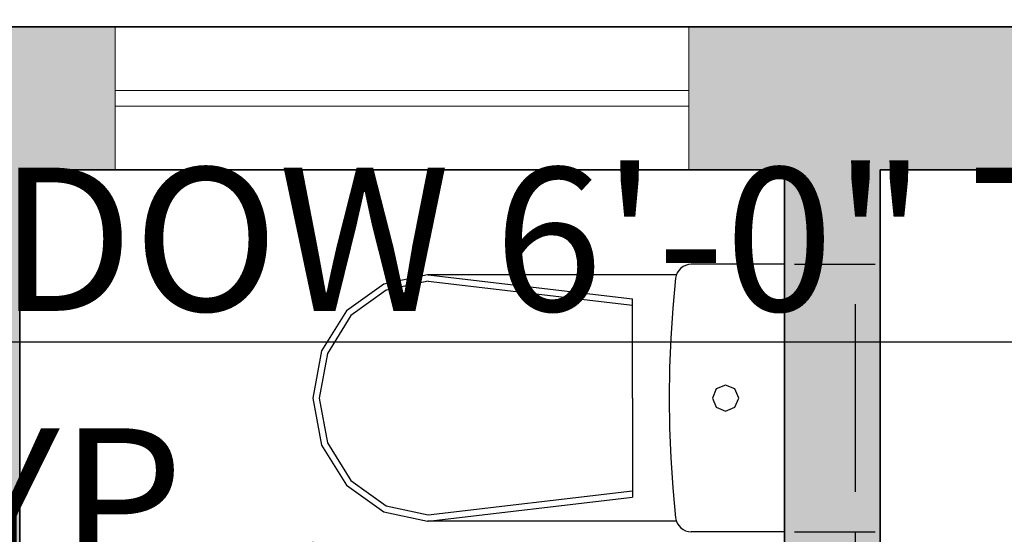
# Model space of a CAD drawing. Units: inches. Extents: x 2831 to 4250, y 1103 to 1797.
# Tile 7 of 15: x 3614 to 3676, y 1658 to 1690. Entities that reach past the tile are written whole.
import ezdxf

# ---------------------------------------------------------------- set-up
doc = ezdxf.new("R2010")
doc.units = ezdxf.units.IN
for name, color, linetype, lineweight in [('A-ANNO-DIMS', 2, 'Continuous', 18), ('A-WALL', 7, 'Continuous', 35), ('A-WALL-PATT', 252, 'Continuous', 13), ('window', 130, 'Continuous', 18), ('Сантехника', 9, 'Continuous', 18)]:
    doc.layers.add(name, color=color, linetype=linetype, lineweight=lineweight)
doc.layers.add('SANTEH', color=7, linetype='Continuous')
doc.styles.get("Standard").update_dxf_attribs({"font": 'arial.ttf'})
doc.dimstyles.new('ISO-25', dxfattribs={"dimtxt": 9, "dimasz": 2.5, "dimexe": 1.25, "dimexo": 0.625, "dimtad": 1, "dimdec": 1, "dimlunit": 3, "dimtxsty": 'Standard', "dimcen": 2.5, "dimadec": 0, "dimazin": 0, "dimtfac": 1, "dimtdec": 1, "dimtmove": 0, "dimatfit": 3, "dimfxl": 1, "dimarcsym": 0})

# ---------------------------------------------------------------- blocks, each defined once
blk = doc.blocks.new('WC 2 Symb_109')
at = {"layer": 'SANTEH'}
for p, q in [((0, 0), (0, 380)), ((0, 380), (132.4, 380)), ((153.6, 364.9), (506.8, 364.9)), ((506.3, 364.9), (215.7, 330.9)), ((506.3, 356), (215.7, 322)), ((215.7, 190), (215.7, 330.9)), ((215.7, 190), (215.7, 49.1)), ((506.3, 24), (215.7, 58)), ((506.3, 15.1), (215.7, 49.1)), ((153.8, 15.1), (506.8, 15.1)), ((0, 0), (132.4, 0))]:
    blk.add_line(p, q, dxfattribs=at)
for points in [[(154.6, 360.1), (153.9, 364.1), (152.3, 367.9), (150.2, 371.3), (147.4, 374.3), (144.1, 376.7), (140.5, 378.5), (136.5, 379.6), (132.4, 380)], [(506.8, 15.1), (569.2, 28.4), (622.2, 66.3), (657.6, 123.1), (670, 190), (657.6, 256.9), (622.2, 313.7), (569.2, 351.6), (506.8, 364.9)], [(154.6, 19.7), (158.6, 62.1), (161.4, 104.7), (163.1, 147.3), (163.7, 189.9), (163.1, 232.5), (161.4, 275.1), (158.6, 317.7), (154.6, 360.1)], [(506.3, 24), (565.5, 36.6), (615.7, 72.6), (649.2, 126.5), (661, 190), (649.2, 253.5), (615.7, 307.4), (565.5, 343.4), (506.3, 356)], [(132.4, 0), (136.5, 0.4), (140.4, 1.5), (144.1, 3.2), (147.3, 5.6), (150.1, 8.6), (152.3, 12), (153.8, 15.7), (154.6, 19.7)]]:
    blk.add_lwpolyline(points, dxfattribs=at)
blk.add_lwpolyline([(83.6, 208.5), (70.4, 203.1), (64.9, 190), (70.4, 176.9), (83.6, 171.5), (96.8, 176.9), (102.2, 190), (96.8, 203.1)], close=True, dxfattribs=at)
blk = doc.blocks.new('WIN-36IN')
for p, q in [((0, 36), (9, 36)), ((4, 0), (4, 36)), ((5, 0), (5, 36)), ((0, 0), (9, 0))]:
    blk.add_line(p, q)
blk = doc.blocks.new('*D77')
at = {"layer": 'A-ANNO-DIMS', "color": 0, "lineweight": -2, "transparency": 16777216}
for p, q in [((3512.227, 1679.888), (3512.227, 1668.463)), ((3584.227, 1679.888), (3584.227, 1668.463)), ((3514.727, 1669.713), (3581.727, 1669.713)), ((3584.227, 1669.713), (3701.864, 1669.713))]:
    blk.add_line(p, q, dxfattribs=at)
at = {"layer": 'A-ANNO-DIMS', "color": 0, "transparency": 16777216}
for points in [[(3514.727, 1670.13), (3514.727, 1669.297), (3512.227, 1669.713)], [(3581.727, 1670.13), (3581.727, 1669.297), (3584.227, 1669.713)]]:
    blk.add_solid(points, dxfattribs=at)
at = {"layer": 'Defpoints', "color": 0, "transparency": 16777216}
for p in [(3512.227, 1680.513), (3584.227, 1680.513), (3584.227, 1669.713)]:
    blk.add_point(p, dxfattribs=at)
at = {"layer": 'A-ANNO-DIMS', "color": 0, "transparency": 16777216, "insert": (3644.295, 1674.995), "char_height": 9, "attachment_point": 5}
blk.add_mtext('WINDOW 6\'-0" TYP.', dxfattribs=at)
blk = doc.blocks.new('*D89')
at = {"layer": 'A-ANNO-DIMS', "color": 0, "lineweight": -2, "transparency": 16777216}
for p, q in [((3632.619, 1657.173), (3632.619, 1652.107)), ((3662.227, 1657.173), (3662.227, 1652.107)), ((3632.619, 1653.357), (3528.23, 1653.357)), ((3659.727, 1653.357), (3635.119, 1653.357))]:
    blk.add_line(p, q, dxfattribs=at)
at = {"layer": 'A-ANNO-DIMS', "color": 0, "transparency": 16777216}
for points in [[(3635.119, 1653.773), (3635.119, 1652.94), (3632.619, 1653.357)], [(3659.727, 1653.773), (3659.727, 1652.94), (3662.227, 1653.357)]]:
    blk.add_solid(points, dxfattribs=at)
at = {"layer": 'Defpoints', "color": 0, "transparency": 16777216}
for p in [(3632.619, 1657.798), (3662.227, 1657.798), (3632.619, 1653.357)]:
    blk.add_point(p, dxfattribs=at)
at = {"layer": 'A-ANNO-DIMS', "color": 0, "transparency": 16777216, "insert": (3579.175, 1658.635), "char_height": 9, "attachment_point": 5}
blk.add_mtext('WC 2\'-5 1/2" TYP.', dxfattribs=at)
blk = doc.blocks.new('*D90')
at = {"layer": 'A-ANNO-DIMS', "color": 0, "lineweight": -2, "transparency": 16777216}
for p, q in [((3662.852, 1674.59), (3667.918, 1674.59)), ((3666.668, 1672.09), (3666.668, 1660.298)), ((3662.852, 1657.798), (3667.918, 1657.798)), ((3666.668, 1657.798), (3666.668, 1600.035))]:
    blk.add_line(p, q, dxfattribs=at)
at = {"layer": 'A-ANNO-DIMS', "color": 0, "transparency": 16777216}
for points in [[(3666.251, 1672.09), (3667.084, 1672.09), (3666.668, 1674.59)], [(3666.251, 1660.298), (3667.084, 1660.298), (3666.668, 1657.798)]]:
    blk.add_solid(points, dxfattribs=at)
at = {"layer": 'Defpoints', "color": 0, "transparency": 16777216}
for p in [(3662.227, 1674.59), (3662.227, 1657.798), (3666.668, 1657.798)]:
    blk.add_point(p, dxfattribs=at)
at = {"layer": 'A-ANNO-DIMS', "color": 0, "transparency": 16777216, "insert": (3661.448, 1627.666), "char_height": 9, "attachment_point": 5, "rotation": 90}
blk.add_mtext('1\'-5" TYP.', dxfattribs=at)

msp = doc.modelspace()

# ---------------------------------------------------------------- hatches: boundary and pattern name
at = {"layer": 'A-WALL-PATT'}
h = msp.add_hatch(color=256, dxfattribs=at)
h.dxf.hatch_style = 1
h.paths.add_polyline_path([(3479.227, 1418.513), (3488.227, 1418.513), (3488.227, 1426.809), (3488.227, 1460.513), (3588.227, 1460.513), (3588.227, 1466.513), (3488.227, 1466.513), (3488.227, 1470.513), (3479.227, 1470.513)])
h.paths.add_polyline_path([(3488.227, 1506.513), (3488.227, 1512.513), (3479.227, 1512.513), (3479.227, 1506.513)])
h.paths.add_polyline_path([(3488.227, 1370.513), (3479.227, 1370.513), (3479.227, 1319.513), (3521.227, 1319.513), (3521.227, 1328.513), (3488.227, 1328.513)])
h.paths.add_polyline_path([(3794.227, 1319.513), (3794.227, 1247.513), (3614.227, 1247.513), (3614.227, 1242.513), (3803.227, 1242.513), (3803.227, 1328.513), (3767.227, 1328.513), (3767.227, 1394.513), (3758.227, 1394.513), (3758.227, 1328.513), (3635.227, 1328.513), (3635.227, 1460.513), (3637.227, 1460.513), (3637.227, 1466.513), (3624.227, 1466.513), (3624.227, 1460.513), (3626.227, 1460.513), (3626.227, 1328.513), (3593.227, 1328.513), (3593.227, 1319.513)])
h.paths.add_polyline_path([(3758.227, 1460.513), (3758.227, 1442.513), (3767.227, 1442.513), (3767.227, 1460.513), (3783.227, 1460.513), (3783.227, 1492.513), (3774.227, 1492.513), (3774.227, 1466.513), (3761.32, 1466.513), (3726.227, 1466.513), (3726.227, 1468.513), (3720.227, 1468.513), (3720.227, 1466.513), (3673.227, 1466.513), (3673.227, 1460.513)])
h.paths.add_polyline_path([(3597.627, 1698.243), (3687.215, 1698.243), (3687.215, 1717.459), (3597.627, 1717.459)], flags=9)
h.paths.add_polyline_path([(3776.749, 1438.286), (3776.749, 1360.767), (3795.966, 1360.767), (3795.966, 1438.286)], flags=25)
h.paths.add_polyline_path([(3453.373, 1482.946), (3453.373, 1401.852), (3472.59, 1401.852), (3472.59, 1482.946)], flags=9)
h.paths.add_polyline_path([(3506.208, 1267.098), (3560.706, 1267.098), (3560.706, 1293.711), (3506.208, 1293.711)], flags=9)
h.paths.add_polyline_path([(3760.502, 1579.698), (3798.745, 1579.698), (3798.745, 1602.509), (3760.502, 1602.509)], flags=9)
h.paths.add_polyline_path([(3617.004, 1637.953), (3659.123, 1637.953), (3659.123, 1660.764), (3617.004, 1660.764)], flags=9)
h.paths.add_polyline_path([(3679.387, 1612.632), (3728.455, 1612.632), (3728.455, 1639.245), (3679.387, 1639.245)], flags=9)
h.paths.add_polyline_path([(3731.075, 1499.721), (3773.194, 1499.721), (3773.194, 1522.532), (3731.075, 1522.532)], flags=9)
h.paths.add_polyline_path([(3652.819, 1496.485), (3701.947, 1496.485), (3701.947, 1523.098), (3652.819, 1523.098)], flags=9)
h.paths.add_polyline_path([(3550.367, 1510.971), (3604.502, 1510.971), (3604.502, 1537.584), (3550.367, 1537.584)], flags=9)
h.paths.add_polyline_path([(3514.446, 1612.632), (3570.67, 1612.632), (3570.67, 1639.245), (3514.446, 1639.245)], flags=9)
h = msp.add_hatch(color=256, dxfattribs=at)
h.dxf.hatch_style = 1
h.paths.add_polyline_path([(3783.227, 1560.513), (3767.227, 1560.513), (3767.227, 1572.513), (3761.227, 1572.513), (3758.227, 1572.513), (3758.227, 1560.513), (3488.227, 1560.513), (3488.227, 1562.513), (3485.227, 1562.513), (3479.227, 1562.513), (3479.227, 1552.513), (3485.227, 1552.513), (3488.227, 1552.513), (3488.227, 1554.513), (3642.227, 1554.513), (3642.227, 1498.513), (3648.227, 1498.513), (3648.227, 1554.513), (3720.227, 1554.513), (3720.227, 1498.513), (3726.227, 1498.513), (3726.227, 1554.513), (3774.227, 1554.513), (3774.227, 1528.513), (3783.227, 1528.513)])
h.paths.add_polyline_path([(3767.227, 1689.513), (3728.227, 1689.513), (3728.227, 1680.513), (3758.227, 1680.513), (3758.227, 1602.513), (3767.227, 1602.513)])
h.paths.add_polyline_path([(3680.227, 1689.513), (3656.227, 1689.513), (3656.227, 1680.513), (3662.227, 1680.513), (3662.227, 1608.513), (3644.227, 1608.513), (3644.227, 1602.513), (3668.227, 1602.513), (3668.227, 1680.513), (3680.227, 1680.513)])
h.paths.add_polyline_path([(3620.227, 1689.513), (3584.227, 1689.513), (3584.227, 1680.513), (3608.227, 1680.513), (3608.227, 1602.513), (3614.227, 1602.513), (3614.227, 1608.513), (3614.227, 1638.513), (3614.227, 1680.513), (3620.227, 1680.513)])
h.paths.add_polyline_path([(3512.227, 1689.513), (3479.227, 1689.513), (3479.227, 1665.513), (3488.227, 1665.513), (3488.227, 1680.513), (3512.227, 1680.513)])
h.paths.add_polyline_path([(3488.227, 1617.513), (3479.227, 1617.513), (3479.227, 1602.513), (3485.227, 1602.513), (3488.227, 1602.513)])

# ---------------------------------------------------------------- linework, layer by layer
at = {"layer": 'A-WALL'}
for p, q in [((3479.227, 1689.513), (3803.227, 1689.513)), ((3614.227, 1602.513), (3614.227, 1680.513)), ((3614.227, 1680.513), (3662.227, 1680.513)), ((3662.227, 1608.513), (3662.227, 1680.513)), ((3668.227, 1602.513), (3668.227, 1680.513)), ((3668.227, 1680.513), (3758.227, 1680.513))]:
    msp.add_line(p, q, dxfattribs=at)

# ---------------------------------------------------------------- block references
at = {"layer": 'window', "rotation": 89.99999999999523}
msp.add_blockref('WIN-36IN', (3656.227, 1680.513), dxfattribs=at)
at = {"layer": 'Сантехника', "xscale": 0.0441898926459964, "yscale": 0.0441898926459964, "zscale": 0.0441898926459964, "rotation": 180}
msp.add_blockref('WC 2 Symb_109', (3662.227, 1674.59), dxfattribs=at)

# ---------------------------------------------------------------- dimensions: what is measured, and where the dimension line sits
at = {"layer": 'A-ANNO-DIMS'}
dim = msp.add_linear_dim(base=(3584.227, 1669.713), p1=(3512.227, 1680.513), p2=(3584.227, 1680.513), text='WINDOW <> TYP.', dimstyle='ISO-25', override={"dimdec": 1, "dimlfac": 1, "dimrnd": 0, "dimzin": 1, "dimdsep": 46, "dimlunit": 4, "dimfrac": 2}, dxfattribs=at)
dim.commit()
dim.dimension.update_dxf_attribs({"geometry": '*D77', "text_midpoint": (3644.295, 1674.995)})
for base, p1, p2, angle, text, picture, middle in [((3632.619, 1653.357), (3662.227, 1657.798), (3632.619, 1657.798), 180, 'WC <> TYP.', '*D89', (3579.175, 1658.635)), ((3666.668, 1657.798), (3662.227, 1674.59), (3662.227, 1657.798), 270, '<> TYP.', '*D90', (3661.448, 1627.666))]:
    dim = msp.add_linear_dim(base=base, p1=p1, p2=p2, angle=angle, text=text, dimstyle='ISO-25', override={"dimdec": 1, "dimlfac": 1, "dimrnd": 0, "dimzin": 1, "dimdsep": 46, "dimlunit": 4, "dimfrac": 2}, dxfattribs=at)
    dim.commit()
    dim.dimension.update_dxf_attribs({"geometry": picture, "text_midpoint": middle})

doc.saveas('drawing.dxf')
